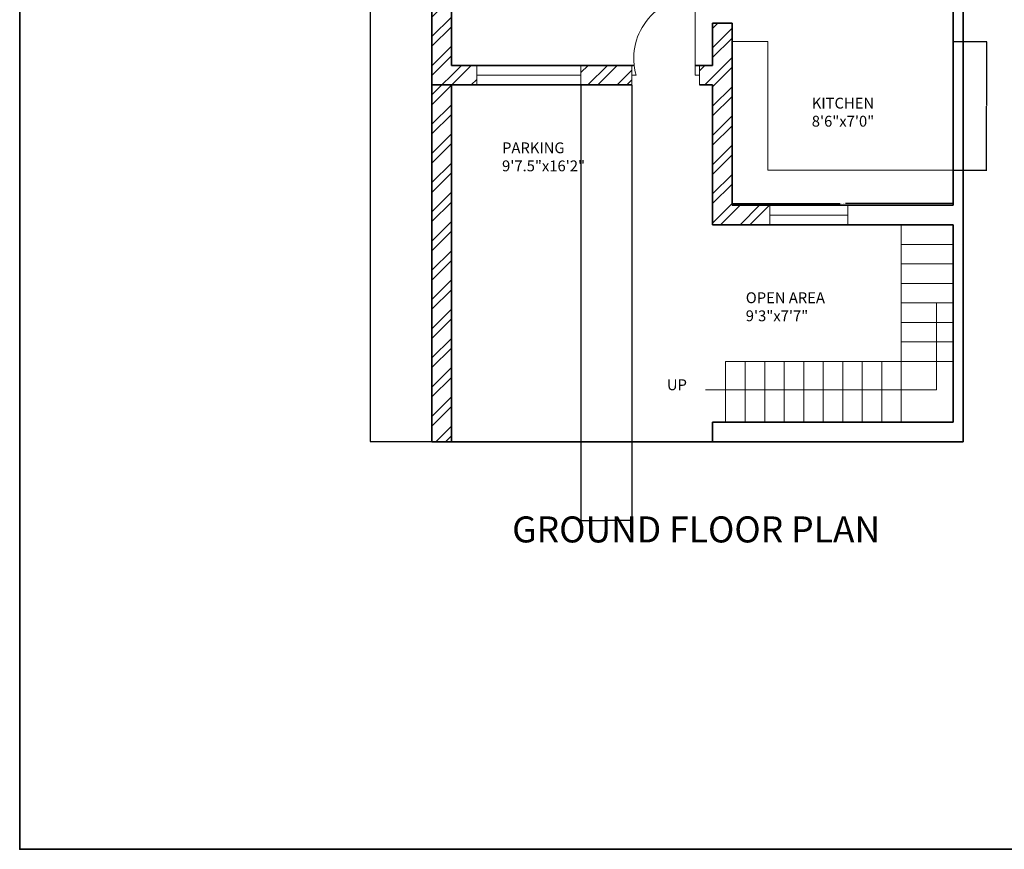
# Model space of a CAD drawing. Units: inches. Extents: x 1850 to 3445, y 1558 to 2756.
# Tile 1 of 13: x 1850 to 2304, y 1558 to 1940. Entities that reach past the tile are written whole.
import ezdxf

# ---------------------------------------------------------------- set-up
doc = ezdxf.new("R2010")
doc.units = ezdxf.units.IN
for name, color, linetype, lineweight in [('A-ANNO-DIMS', 2, 'Continuous', 18), ('A-ANNO-TEXT', 7, 'Continuous', 18), ('A-ANNO-TTLB', 7, 'Continuous', 35), ('A-AREA-IDEN', 7, 'Continuous', 18), ('A-DOOR', 3, 'Continuous', 18), ('A-FLOR-CASE', 8, 'Continuous', 18), ('A-FLOR-STRS', 7, 'Continuous', 18), ('A-GLAZ', 4, 'Continuous', 18), ('A-WALL', 7, 'Continuous', 35), ('A-WALL-PATT', 252, 'Continuous', 13)]:
    doc.layers.add(name, color=color, linetype=linetype, lineweight=lineweight)
doc.styles.get("Standard").update_dxf_attribs({"font": 'arial.ttf'})
doc.dimstyles.get("Standard").update_dxf_attribs({"dimtxt": 0.18, "dimasz": 0.18, "dimexe": 0.18, "dimexo": 0.0625, "dimgap": 0.09, "dimtad": 0, "dimtih": 1, "dimtoh": 1, "dimdec": 4, "dimzin": 0, "dimdsep": 46, "dimtxsty": 'Standard', "dimcen": 0.09, "dimadec": 0, "dimazin": 0, "dimtfac": 1, "dimtdec": 4, "dimtofl": 0, "dimtmove": 0, "dimatfit": 3, "dimfxl": 1, "dimtolj": 1, "dimtzin": 0, "dimarcsym": 0})

# ---------------------------------------------------------------- blocks, each defined once
blk = doc.blocks.new('WIN-48-W9')
for p, q in [((0, 9), (0, 0)), ((48, 4.5), (48, 9)), ((48, 9), (48, 0)), ((0, 0), (0, 4.5)), ((0, 4.5), (48, 4.5))]:
    blk.add_line(p, q)
blk = doc.blocks.new('WIN-36-W9')
for p, q in [((0, 9), (0, 0)), ((36, 4.5), (36, 9)), ((36, 9), (36, 0)), ((0, 0), (0, 4.5)), ((0, 4.5), (36, 4.5))]:
    blk.add_line(p, q)
blk = doc.blocks.new('DOOR-ENTRY-GROUND')
for p, q in [((29.19, 4.5), (29.19, 40.5)), ((0, 9), (0, 2.33)), ((31.19, 9), (31.19, 0)), ((0, 0), (0, 4.46)), ((0, 4.46), (2, 4.46)), ((0, 2.33), (0, 0)), ((31.19, 4.5), (29.19, 4.5)), ((31.19, 0), (31.19, 4.5))]:
    blk.add_line(p, q)
blk.add_arc((29.19, 12.22), 28.28, 90, 195.9327)
blk = doc.blocks.new('STAIR-L-GROUND')
for p, q in [((81, 28), (81, 91)), ((105, 91), (81, 91)), ((105, 82), (81, 82)), ((105, 73), (81, 73)), ((105, 64), (81, 64)), ((105, 55), (81, 55)), ((105, 46), (81, 46)), ((105, 37), (81, 37)), ((0, 0), (0, 28)), ((0, 28), (105, 28)), ((9, 0), (9, 28)), ((18, 0), (18, 28)), ((27, 0), (27, 28)), ((36, 0), (36, 28)), ((45, 0), (45, 28)), ((54, 0), (54, 28)), ((63, 0), (63, 28)), ((102.7, 28), (72, 28)), ((72, 0), (72, 28)), ((81, 0), (81, 28))]:
    blk.add_line(p, q)
blk = doc.blocks.new('COUNTER-L-GROUND')
for p, q in [((0, 59.33), (16.51, 59.33)), ((16.51, 59.33), (16.51, 0)), ((16.51, 0), (102, 0))]:
    blk.add_line(p, q)
blk = doc.blocks.new('*D72')
at = {"layer": 'A-ANNO-DIMS', "color": 0, "lineweight": -2, "transparency": 16777216}
for p, q in [((2178.77, 1870.8), (2178.77, 1855.38)), ((2280.77, 1870.8), (2280.77, 1855.38)), ((2178.95, 1855.56), (2228.52, 1855.56)), ((2280.59, 1855.56), (2231.03, 1855.56))]:
    blk.add_line(p, q, dxfattribs=at)
at = {"layer": 'A-ANNO-DIMS', "color": 0, "transparency": 16777216}
for points in [[(2178.95, 1855.59), (2178.95, 1855.53), (2178.77, 1855.56)], [(2280.59, 1855.59), (2280.59, 1855.53), (2280.77, 1855.56)]]:
    blk.add_solid(points, dxfattribs=at)
at = {"layer": 'Defpoints', "color": 0, "transparency": 16777216}
for p in [(2178.77, 1870.86), (2280.77, 1870.86), (2280.77, 1855.56)]:
    blk.add_point(p, dxfattribs=at)
at = {"layer": 'A-ANNO-DIMS', "color": 0, "transparency": 16777216, "insert": (2229.77, 1855.56), "char_height": 0.18, "attachment_point": 5}
blk.add_mtext('\\A1;COUNTER 102 TYP.', dxfattribs=at)
blk = doc.blocks.new('*D73')
at = {"layer": 'A-ANNO-DIMS', "color": 0, "lineweight": -2, "transparency": 16777216}
for p, q in [((2280.83, 1930.19), (2296.25, 1930.19)), ((2296.07, 1930.01), (2296.07, 1900.71)), ((2296.07, 1871.04), (2296.07, 1900.35)), ((2280.83, 1870.86), (2296.25, 1870.86))]:
    blk.add_line(p, q, dxfattribs=at)
at = {"layer": 'A-ANNO-DIMS', "color": 0, "transparency": 16777216}
for points in [[(2296.04, 1930.01), (2296.1, 1930.01), (2296.07, 1930.19)], [(2296.04, 1871.04), (2296.1, 1871.04), (2296.07, 1870.86)]]:
    blk.add_solid(points, dxfattribs=at)
at = {"layer": 'Defpoints', "color": 0, "transparency": 16777216}
for p in [(2280.77, 1930.19), (2296.07, 1930.19), (2280.77, 1870.86)]:
    blk.add_point(p, dxfattribs=at)
at = {"layer": 'A-ANNO-DIMS', "color": 0, "transparency": 16777216, "insert": (2296.07, 1900.53), "char_height": 0.18, "attachment_point": 5}
blk.add_mtext('\\A1;59 TYP.', dxfattribs=at)
blk = doc.blocks.new('*D81')
at = {"layer": 'A-ANNO-DIMS', "color": 0, "lineweight": -2, "transparency": 16777216}
for p, q in [((2040.21, 2216.18), (2011.84, 2216.18)), ((2012.02, 2216), (2012.02, 1981.12)), ((2012.02, 1745.86), (2012.02, 1980.75)), ((2040.21, 1745.68), (2011.84, 1745.68))]:
    blk.add_line(p, q, dxfattribs=at)
at = {"layer": 'A-ANNO-DIMS', "color": 0, "transparency": 16777216}
for points in [[(2011.99, 2216), (2012.05, 2216), (2012.02, 2216.18)], [(2011.99, 1745.86), (2012.05, 1745.86), (2012.02, 1745.68)]]:
    blk.add_solid(points, dxfattribs=at)
at = {"layer": 'Defpoints', "color": 0, "transparency": 16777216}
for p in [(2012.02, 2216.18), (2040.27, 2216.18), (2040.27, 1745.68)]:
    blk.add_point(p, dxfattribs=at)
at = {"layer": 'A-ANNO-DIMS', "color": 0, "transparency": 16777216, "insert": (2012.02, 1980.93), "char_height": 0.18, "attachment_point": 5}
blk.add_mtext('\\A1;470.5', dxfattribs=at)
blk = doc.blocks.new('*D84')
at = {"layer": 'A-ANNO-DIMS', "color": 0, "lineweight": -2, "transparency": 16777216}
for p, q in [((2108.95, 1910.15), (2108.95, 1709.25)), ((2132.49, 1910.15), (2132.49, 1709.25)), ((2109.13, 1709.43), (2120.26, 1709.43)), ((2132.31, 1709.43), (2121.19, 1709.43))]:
    blk.add_line(p, q, dxfattribs=at)
at = {"layer": 'A-ANNO-DIMS', "color": 0, "transparency": 16777216}
for points in [[(2109.13, 1709.46), (2109.13, 1709.4), (2108.95, 1709.43)], [(2132.31, 1709.46), (2132.31, 1709.4), (2132.49, 1709.43)]]:
    blk.add_solid(points, dxfattribs=at)
at = {"layer": 'Defpoints', "color": 0, "transparency": 16777216}
for p in [(2108.95, 1910.22), (2132.49, 1910.22), (2132.49, 1709.43)]:
    blk.add_point(p, dxfattribs=at)
at = {"layer": 'A-ANNO-DIMS', "color": 0, "transparency": 16777216, "insert": (2120.72, 1709.43), "char_height": 0.18, "attachment_point": 5}
blk.add_mtext('\\A1;23.546', dxfattribs=at)

msp = doc.modelspace()

# ---------------------------------------------------------------- hatches: boundary and pattern name
at = {"layer": 'A-WALL-PATT'}
h = msp.add_hatch(dxfattribs=at)
h.set_pattern_fill('ANSI32', color=256)
h.paths.add_polyline_path([(2519.5556, 1907.3936), (2523.9987, 1907.3936), (2523.9987, 1916.3936), (2519.5556, 1916.3936), (2515.0556, 1916.3936), (2510.5556, 1916.3936), (2510.5556, 1907.3936), (2515.0556, 1907.3936), (2515.0556, 1742.1843), (2515.0556, 1737.6843), (2596.0556, 1737.6843), (2596.0556, 1976.4962), (2591.5556, 1976.4962), (2591.5556, 1916.3936), (2561.2666, 1916.3936), (2561.2666, 1907.3936), (2591.5556, 1907.3936), (2591.5556, 1746.6843), (2519.5556, 1746.6843)])
h.paths.add_polyline_path([(2076.6481, 2211.6843), (2076.6481, 2216.1843), (2040.2715, 2216.1843), (2040.2715, 2175.83), (2044.7715, 2175.83), (2049.2715, 2175.83), (2049.2715, 2207.1843), (2076.6481, 2207.1843)])
h.paths.add_polyline_path([(2211.7715, 2216.1843), (2136.6481, 2216.1843), (2136.6481, 2207.1843), (2211.7715, 2207.1843)])
h.paths.add_polyline_path([(2285.2715, 2154.1843), (2250.6169, 2154.1843), (2250.6169, 2149.6843), (2280.7715, 2149.6843), (2280.7715, 2075.1843), (2236.3632, 2075.1843), (2236.3632, 2070.6843), (2285.2715, 2070.6843)])
h.paths.add_polyline_path([(2228.3485, 2154.1843), (2207.2715, 2154.1843), (2207.2715, 2075.1843), (2201.9819, 2075.1843), (2201.9819, 2070.6843), (2215.4663, 2070.6843), (2215.4663, 2072.9343), (2215.4663, 2075.1843), (2211.7715, 2075.1843), (2211.7715, 2149.6843), (2228.3485, 2149.6843)])
h.paths.add_polyline_path([(2049.2715, 2115.83), (2040.2715, 2115.83), (2040.2715, 2042.8465), (2049.2715, 2042.8465), (2049.2715, 2070.6843), (2168.6057, 2070.6843), (2168.6057, 2072.9343), (2168.6057, 2075.1843), (2049.2715, 2075.1843)])
h.paths.add_polyline_path([(2049.2715, 1982.8465), (2040.2715, 1982.8465), (2040.2715, 1910.2175), (2060.9481, 1910.2175), (2060.9481, 1914.7175), (2060.9481, 1919.2175), (2049.2715, 1919.2175)])
h.paths.add_polyline_path([(2132.4938, 1919.2175), (2108.9481, 1919.2175), (2108.9481, 1910.2175), (2132.4938, 1910.2175), (2132.4938, 1914.6749)])
h.paths.add_polyline_path([(2178.7715, 1938.6843), (2169.7715, 1938.6843), (2169.7715, 1919.2175), (2163.687, 1919.2175), (2163.687, 1910.2175), (2169.7715, 1910.2175), (2169.7715, 1854.6843), (2169.7715, 1845.6843), (2196.1287, 1845.6843), (2196.1287, 1850.1843), (2196.1287, 1854.6843), (2178.7715, 1854.6843)])
h.paths.add_polyline_path([(2049.2715, 1910.2175), (2040.2715, 1910.2175), (2040.2715, 1745.6843), (2049.2715, 1745.6843)])
h.paths.add_polyline_path([(2146.8861, 1766.7204), (2159.0894, 1766.7204), (2159.0894, 1777.0239), (2146.8861, 1777.0239)], flags=9)
h.paths.add_polyline_path([(2183.4664, 1798.4016), (2226.7338, 1798.4016), (2226.7338, 1817.0589), (2183.4664, 1817.0589)], flags=9)
h.paths.add_polyline_path([(2070.863, 1867.537), (2109.9796, 1867.537), (2109.9796, 1886.1943), (2070.863, 1886.1943)], flags=9)

# ---------------------------------------------------------------- linework, layer by layer
at = {"layer": 'A-ANNO-TTLB'}
msp.add_lwpolyline([(1850.1793, 2756.3177), (3445.2682, 2756.3177), (3445.2682, 1557.7728), (1850.1793, 1557.7728)], close=True, dxfattribs=at)
at = {"layer": 'A-FLOR-STRS'}
for p, q in [((2272.9405, 1769.5741), (2272.9405, 1809.6843)), ((2166.452, 1769.5741), (2272.9405, 1769.5741))]:
    msp.add_line(p, q, dxfattribs=at)
at = {"layer": 'A-WALL'}
for p, q in [((2040.2715, 2216.1843), (2040.2715, 1745.6843)), ((2285.2715, 2207.1843), (2285.2715, 1745.6843)), ((2049.2715, 2070.6843), (2049.2715, 1919.2175)), ((2280.7715, 2070.6843), (2280.7715, 1854.6843)), ((2169.7715, 1938.6843), (2178.7715, 1938.6843)), ((2178.7715, 1938.6843), (2169.7715, 1938.6843)), ((2169.7715, 1938.6843), (2169.7715, 1919.2175)), ((2178.7715, 1854.6843), (2178.7715, 1938.6843)), ((2049.2715, 1919.2175), (2133.5914, 1919.2175)), ((2161.687, 1919.2175), (2169.7715, 1919.2175)), ((2132.4938, 1910.2175), (2040.2715, 1910.2175)), ((2049.2715, 1910.2175), (2049.2715, 1745.6843)), ((2169.7715, 1910.2175), (2163.687, 1910.2175)), ((2169.7715, 1910.2175), (2169.7715, 1854.6843)), ((2169.7715, 1854.6843), (2169.7715, 1845.6843)), ((2280.7715, 1854.6843), (2178.7715, 1854.6843)), ((2169.7715, 1845.6843), (2280.7715, 1845.6843)), ((2280.7715, 1845.6843), (2280.7715, 1754.6843)), ((2280.7715, 1845.6843), (2280.7715, 1754.6843)), ((2280.7715, 1754.6843), (2169.7715, 1754.6843)), ((2169.7715, 1754.6843), (2169.7715, 1745.6843)), ((2169.7715, 1745.6843), (2040.2715, 1745.6843)), ((2169.7715, 1745.6843), (2280.7715, 1745.6843)), ((2280.7715, 1745.6843), (2285.2715, 1745.6843))]:
    msp.add_line(p, q, dxfattribs=at)

# ---------------------------------------------------------------- block references
at = {"layer": 'A-DOOR'}
msp.add_blockref('DOOR-ENTRY-GROUND', (2132.494, 1910.217), dxfattribs=at)
at = {"layer": 'A-FLOR-CASE'}
msp.add_blockref('COUNTER-L-GROUND', (2178.771, 1870.864), dxfattribs=at)
at = {"layer": 'A-FLOR-STRS'}
msp.add_blockref('STAIR-L-GROUND', (2175.771, 1754.684), dxfattribs=at)
at = {"layer": 'A-GLAZ'}
for name, p in [('WIN-48-W9', (2060.948, 1910.217)), ('WIN-36-W9', (2196.129, 1845.684))]:
    msp.add_blockref(name, p, dxfattribs=at)

# ---------------------------------------------------------------- texts
at = {"layer": 'A-ANNO-TEXT', "attachment_point": 1}
for s, width, insert, char_height in [('UP', 23.427973, (2148.6852, 1774.4506), 5), ('GROUND FLOOR PLAN', 287.616418, (2077.3192, 1711.2535), 12)]:
    msp.add_mtext_dynamic_manual_height_columns(s, width=width, gutter_width=12.5, heights=[0], dxfattribs=dict(at, insert=insert, char_height=char_height))
at = {"layer": 'A-AREA-IDEN', "char_height": 5, "attachment_point": 1}
for s, width, insert in [('KITCHEN\\P8\'6"x7\'0"', 84.206423, (2215.4867, 1904.3015)), ('PARKING\\P9\'7.5"x16\'2"', 110.113672, (2072.6519, 1883.7063)), ('OPEN AREA\\P9\'3"x7\'7"', 100.217422, (2185.054, 1814.5743))]:
    msp.add_mtext_dynamic_manual_height_columns(s, width=width, gutter_width=12.5, heights=[0], dxfattribs=dict(at, insert=insert))

# ---------------------------------------------------------------- dimensions: what is measured, and where the dimension line sits
at = {"layer": 'A-ANNO-DIMS'}
dim = msp.add_linear_dim(base=(2012.0215, 2216.1843), p1=(2040.2715, 1745.6843), p2=(2040.2715, 2216.1843), angle=90, dimstyle='Standard', override={"dimdec": 1, "dimlfac": 1, "dimrnd": 0, "dimzin": 0, "dimdsep": 46, "dimlunit": 2}, dxfattribs=at)
dim.commit()
dim.dimension.update_dxf_attribs({"geometry": '*D81', "text_midpoint": (2012.0215, 1980.9343)})
dim = msp.add_linear_dim(base=(2296.0715, 1930.195), p1=(2280.7715, 1870.8639), p2=(2280.7715, 1930.195), angle=90, text='<> TYP.', dimstyle='Standard', override={"dimdec": 0, "dimlfac": 1, "dimrnd": 0, "dimzin": 0, "dimdsep": 46, "dimlunit": 2}, dxfattribs=at)
dim.commit()
dim.dimension.update_dxf_attribs({"geometry": '*D73', "text_midpoint": (2296.0715, 1900.5295)})
dim = msp.add_linear_dim(base=(2132.4938, 1709.4343), p1=(2108.9481, 1910.2175), p2=(2132.4938, 1910.2175), dimstyle='Standard', override={"dimdec": 3, "dimlfac": 1, "dimrnd": 0, "dimzin": 0, "dimdsep": 46, "dimlunit": 2}, dxfattribs=at)
dim.commit()
dim.dimension.update_dxf_attribs({"geometry": '*D84', "text_midpoint": (2120.7209, 1709.4343)})
dim = msp.add_linear_dim(base=(2280.7715, 1855.5639), p1=(2178.7715, 1870.8639), p2=(2280.7715, 1870.8639), text='COUNTER <> TYP.', dimstyle='Standard', override={"dimdec": 0, "dimlfac": 1, "dimrnd": 0, "dimzin": 0, "dimdsep": 46, "dimlunit": 2}, dxfattribs=at)
dim.commit()
dim.dimension.update_dxf_attribs({"geometry": '*D72', "text_midpoint": (2229.7715, 1855.5639)})

doc.saveas('drawing.dxf')
